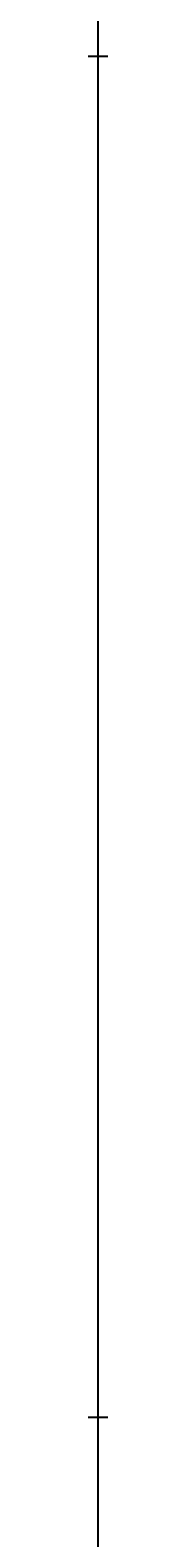
# Model space of a CAD drawing. Units: inches. Extents: x 35362 to 73946, y 43607 to 67532.
# Tile 33 of 134: x 48373 to 48373, y 46091 to 46564. Entities that reach past the tile are written whole.
import ezdxf

# ---------------------------------------------------------------- set-up
doc = ezdxf.new("R2010")
doc.units = ezdxf.units.IN
doc.header["$MEASUREMENT"] = 0
doc.layers.add('A-ANNO-DIMS', color=2, linetype='Continuous', lineweight=18)
doc.styles.get("Standard").update_dxf_attribs({"font": 'arial.ttf'})
doc.dimstyles.get("Standard").update_dxf_attribs({"dimtxt": 0.18, "dimasz": 0.18, "dimexe": 0.18, "dimexo": 0.0625, "dimgap": 0.09, "dimtad": 0, "dimtih": 1, "dimtoh": 1, "dimdec": 4, "dimzin": 0, "dimdsep": 46, "dimtxsty": 'Standard', "dimcen": 0.09, "dimadec": 0, "dimazin": 0, "dimtfac": 1, "dimtdec": 4, "dimtofl": 0, "dimtmove": 0, "dimatfit": 3, "dimfxl": 1, "dimtolj": 1, "dimtzin": 0, "dimarcsym": 0})

# ---------------------------------------------------------------- blocks, each defined once
blk = doc.blocks.new('*D5')
at = {"layer": 'A-ANNO-DIMS', "color": 0, "lineweight": -2, "transparency": 16777216}
for p, q in [((37121.95, 46919.32), (37121.95, 43606.68)), ((69871.5, 45449.83), (69871.5, 43606.68)), ((37122.13, 43606.86), (53496.29, 43606.86)), ((69871.32, 43606.86), (53497.15, 43606.86))]:
    blk.add_line(p, q, dxfattribs=at)
at = {"layer": 'A-ANNO-DIMS', "color": 0, "transparency": 16777216}
for points in [[(37122.13, 43606.89), (37122.13, 43606.83), (37121.95, 43606.86)], [(69871.32, 43606.89), (69871.32, 43606.83), (69871.5, 43606.86)]]:
    blk.add_solid(points, dxfattribs=at)
at = {"layer": 'Defpoints', "color": 0, "transparency": 16777216}
for p in [(37121.95, 46919.38), (69871.5, 45449.89), (69871.5, 43606.86)]:
    blk.add_point(p, dxfattribs=at)
at = {"layer": 'A-ANNO-DIMS', "color": 0, "transparency": 16777216, "insert": (53496.72, 43606.86), "char_height": 0.18, "attachment_point": 5}
blk.add_mtext('\\A1;32750', dxfattribs=at)
blk = doc.blocks.new('*D11')
at = {"layer": 'A-ANNO-DIMS', "color": 0, "lineweight": -2, "transparency": 16777216}
for p, q in [((47978.66, 56028.77), (47978.66, 43606.68)), ((53109.76, 56028.77), (53109.76, 43606.68)), ((47978.84, 43606.86), (50543.87, 43606.86)), ((53109.58, 43606.86), (50544.55, 43606.86))]:
    blk.add_line(p, q, dxfattribs=at)
at = {"layer": 'A-ANNO-DIMS', "color": 0, "transparency": 16777216}
for points in [[(47978.84, 43606.89), (47978.84, 43606.83), (47978.66, 43606.86)], [(53109.58, 43606.89), (53109.58, 43606.83), (53109.76, 43606.86)]]:
    blk.add_solid(points, dxfattribs=at)
at = {"layer": 'Defpoints', "color": 0, "transparency": 16777216}
for p in [(47978.66, 56028.84), (53109.76, 56028.84), (53109.76, 43606.86)]:
    blk.add_point(p, dxfattribs=at)
at = {"layer": 'A-ANNO-DIMS', "color": 0, "transparency": 16777216, "insert": (50544.21, 43606.86), "char_height": 0.18, "attachment_point": 5}
blk.add_mtext('\\A1;5131', dxfattribs=at)
blk = doc.blocks.new('*D27')
at = {"layer": 'A-ANNO-DIMS', "color": 0, "lineweight": -2, "transparency": 16777216}
for p, q in [((47978.66, 56028.77), (47978.66, 43606.68)), ((48373.49, 53428.96), (48373.49, 43606.68)), ((47978.84, 43606.86), (48175.68, 43606.86)), ((48373.31, 43606.86), (48176.47, 43606.86))]:
    blk.add_line(p, q, dxfattribs=at)
at = {"layer": 'A-ANNO-DIMS', "color": 0, "transparency": 16777216}
for points in [[(47978.84, 43606.89), (47978.84, 43606.83), (47978.66, 43606.86)], [(48373.31, 43606.89), (48373.31, 43606.83), (48373.49, 43606.86)]]:
    blk.add_solid(points, dxfattribs=at)
at = {"layer": 'Defpoints', "color": 0, "transparency": 16777216}
for p in [(47978.66, 56028.84), (48373.49, 53429.02), (48373.49, 43606.86)]:
    blk.add_point(p, dxfattribs=at)
at = {"layer": 'A-ANNO-DIMS', "color": 0, "transparency": 16777216, "insert": (48176.08, 43606.86), "char_height": 0.18, "attachment_point": 5}
blk.add_mtext('\\A1;394.8', dxfattribs=at)
blk = doc.blocks.new('*D67')
at = {"layer": 'A-ANNO-DIMS', "color": 0, "lineweight": -2, "transparency": 16777216}
for p, q in [((56873.54, 53351.53), (35361.77, 53351.53)), ((35361.95, 53351.35), (35361.95, 49400.89)), ((35361.95, 45450.07), (35361.95, 49400.53)), ((53793.58, 45449.89), (35361.77, 45449.89))]:
    blk.add_line(p, q, dxfattribs=at)
at = {"layer": 'A-ANNO-DIMS', "color": 0, "transparency": 16777216}
for points in [[(35361.92, 53351.35), (35361.98, 53351.35), (35361.95, 53351.53)], [(35361.92, 45450.07), (35361.98, 45450.07), (35361.95, 45449.89)]]:
    blk.add_solid(points, dxfattribs=at)
at = {"layer": 'Defpoints', "color": 0, "transparency": 16777216}
for p in [(35361.95, 53351.53), (56873.6, 53351.53), (53793.64, 45449.89)]:
    blk.add_point(p, dxfattribs=at)
at = {"layer": 'A-ANNO-DIMS', "color": 0, "transparency": 16777216, "insert": (35361.95, 49400.71), "char_height": 0.18, "attachment_point": 5}
blk.add_mtext('\\A1;7901.6', dxfattribs=at)
blk = doc.blocks.new('*D76')
at = {"layer": 'A-ANNO-DIMS', "color": 0, "lineweight": -2, "transparency": 16777216}
for p, q in [((54052.84, 46555.29), (35361.77, 46555.29)), ((35361.95, 46555.11), (35361.95, 46342.27)), ((35361.95, 46129.06), (35361.95, 46341.9)), ((53793.58, 46128.88), (35361.77, 46128.88))]:
    blk.add_line(p, q, dxfattribs=at)
at = {"layer": 'A-ANNO-DIMS', "color": 0, "transparency": 16777216}
for points in [[(35361.92, 46555.11), (35361.98, 46555.11), (35361.95, 46555.29)], [(35361.92, 46129.06), (35361.98, 46129.06), (35361.95, 46128.88)]]:
    blk.add_solid(points, dxfattribs=at)
at = {"layer": 'Defpoints', "color": 0, "transparency": 16777216}
for p in [(35361.95, 46555.29), (54052.9, 46555.29), (53793.64, 46128.88)]:
    blk.add_point(p, dxfattribs=at)
at = {"layer": 'A-ANNO-DIMS', "color": 0, "transparency": 16777216, "insert": (35361.95, 46342.09), "char_height": 0.18, "attachment_point": 5}
blk.add_mtext('\\A1;426.4', dxfattribs=at)
blk = doc.blocks.new('*D90')
at = {"layer": 'A-ANNO-DIMS', "color": 0, "lineweight": -2, "transparency": 16777216}
for p, q in [((53707.72, 47291.29), (35361.77, 47291.29)), ((35361.95, 47291.11), (35361.95, 46710.26)), ((35361.95, 46129.06), (35361.95, 46709.9)), ((53793.58, 46128.88), (35361.77, 46128.88))]:
    blk.add_line(p, q, dxfattribs=at)
at = {"layer": 'A-ANNO-DIMS', "color": 0, "transparency": 16777216}
for points in [[(35361.92, 47291.11), (35361.98, 47291.11), (35361.95, 47291.29)], [(35361.92, 46129.06), (35361.98, 46129.06), (35361.95, 46128.88)]]:
    blk.add_solid(points, dxfattribs=at)
at = {"layer": 'Defpoints', "color": 0, "transparency": 16777216}
for p in [(53707.78, 47291.29), (35361.95, 46128.88), (53793.64, 46128.88)]:
    blk.add_point(p, dxfattribs=at)
at = {"layer": 'A-ANNO-DIMS', "color": 0, "transparency": 16777216, "insert": (35361.95, 46710.08), "char_height": 0.18, "attachment_point": 5}
blk.add_mtext('\\A1;1162.4', dxfattribs=at)

msp = doc.modelspace()

# ---------------------------------------------------------------- dimensions: what is measured, and where the dimension line sits
at = {"layer": 'A-ANNO-DIMS'}
for base, p1, p2, override, picture, middle in [((53109.76, 43606.859), (47978.665, 56028.836), (53109.76, 56028.836), {"dimdec": 0, "dimlfac": 1, "dimrnd": 0, "dimzin": 0, "dimdsep": 46, "dimlunit": 2}, '*D11', (50544.212, 43606.859)), ((48373.492, 43606.859), (47978.665, 56028.836), (48373.492, 53429.019), {"dimdec": 1, "dimlfac": 1, "dimrnd": 0, "dimzin": 0, "dimdsep": 46, "dimlunit": 2}, '*D27', (48176.078, 43606.859)), ((69871.496, 43606.859), (37121.949, 46919.381), (69871.496, 45449.894), {"dimdec": 0, "dimlfac": 1, "dimrnd": 0, "dimzin": 0, "dimdsep": 46, "dimlunit": 2}, '*D5', (53496.723, 43606.859))]:
    dim = msp.add_linear_dim(base=base, p1=p1, p2=p2, dimstyle='Standard', override=override, dxfattribs=at)
    dim.commit()
    dim.dimension.update_dxf_attribs({"geometry": picture, "text_midpoint": middle})
for base, p1, p2, picture, middle in [((35361.949, 53351.529), (53793.638, 45449.894), (56873.602, 53351.529), '*D67', (35361.949, 49400.712)), ((35361.949, 46128.878), (53707.781, 47291.285), (53793.638, 46128.878), '*D90', (35361.949, 46710.081)), ((35361.949, 46555.293), (53793.638, 46128.878), (54052.899, 46555.293), '*D76', (35361.949, 46342.086))]:
    dim = msp.add_linear_dim(base=base, p1=p1, p2=p2, angle=90, dimstyle='Standard', override={"dimdec": 1, "dimlfac": 1, "dimrnd": 0, "dimzin": 0, "dimdsep": 46, "dimlunit": 2}, dxfattribs=at)
    dim.commit()
    dim.dimension.update_dxf_attribs({"geometry": picture, "text_midpoint": middle})

doc.saveas('drawing.dxf')
